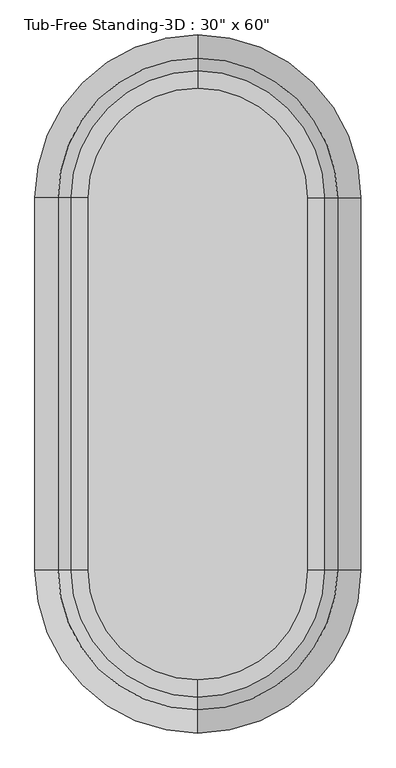
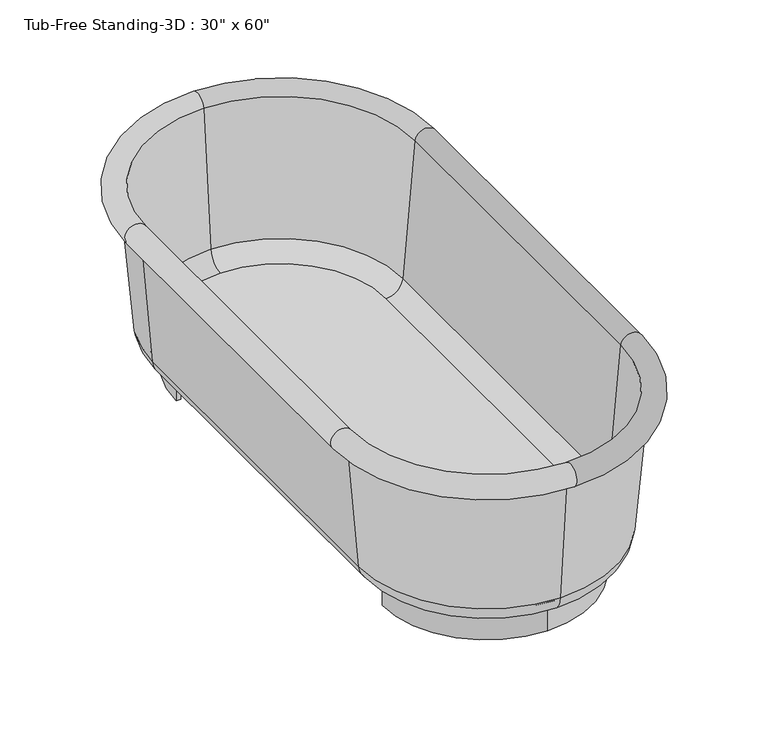
"""IFC4 building model written with IfcOpenShell, lengths in millimetres: flow terminal geometry."""

from ifc_helpers import new_model, si_unit, point, frame, frame_2d, origin, origin_with_axes, place, context, project, spatial, polyline, circle_curve, ellipse_curve, trimmed, segment, composite_curve, outline, extrude, source, transform, mapped, element, save
from ifc_brep_helpers import plane_surface, cylinder_surface, revolved_surface, advanced_brep


def flow_terminal_9fc66f1c(model_context):
    return source(origin(), model_context, "Body", "SolidModel", [
        extrude(outline(composite_curve([segment(trimmed(circle_curve(frame_2d((0.0, 406.4)), 228.6), [point((0.0, 635.0))], [point((-228.6, 406.4))], True, "CARTESIAN"), True, "CONTINUOUS"), segment(polyline([(-228.6, 406.4), (-238.8824236, 406.4)]), True, "CONTINUOUS"), segment(trimmed(circle_curve(frame_2d((0.0, 406.4)), 238.8824236), [point((-238.8824236, 406.4))], [point((0.0, 645.2824236))], False, "CARTESIAN"), True, "CONTINUOUS"), segment(trimmed(circle_curve(frame_2d((0.0, 406.4)), 238.8824236), [point((0.0, 645.2824236))], [point((238.8824236, 406.4))], False, "CARTESIAN"), True, "CONTINUOUS"), segment(polyline([(238.8824236, 406.4), (228.6, 406.4)]), True, "CONTINUOUS"), segment(trimmed(circle_curve(frame_2d((0.0, 406.4)), 228.6), [point((228.6, 406.4))], [point((0.0, 635.0))], True, "CARTESIAN"), True, "CONTINUOUS")], self_intersect=False)), origin_with_axes(), (0.0, 0.0, 1.0), 63.5),
        extrude(outline(composite_curve([segment(trimmed(circle_curve(frame_2d((0.0, -406.4)), 238.8824236), [point((0.0, -645.2824236))], [point((-238.8824236, -406.4))], False, "CARTESIAN"), True, "CONTINUOUS"), segment(polyline([(-238.8824236, -406.4), (-228.6, -406.4)]), True, "CONTINUOUS"), segment(trimmed(circle_curve(frame_2d((0.0, -406.4)), 228.6), [point((-228.6, -406.4))], [point((0.0, -635.0))], True, "CARTESIAN"), True, "CONTINUOUS"), segment(trimmed(circle_curve(frame_2d((0.0, -406.4)), 228.6), [point((0.0, -635.0))], [point((228.6, -406.4))], True, "CARTESIAN"), True, "CONTINUOUS"), segment(polyline([(228.6, -406.4), (238.8824236, -406.4)]), True, "CONTINUOUS"), segment(trimmed(circle_curve(frame_2d((0.0, -406.4)), 238.8824236), [point((238.8824236, -406.4))], [point((0.0, -645.2824236))], False, "CARTESIAN"), True, "CONTINUOUS")], self_intersect=False)), origin_with_axes(), (0.0, 0.0, 1.0), 63.5),
        extrude(outline(composite_curve([segment(polyline([(-238.8824236, -406.4), (-238.8824236, 406.4)]), True, "CONTINUOUS"), segment(trimmed(circle_curve(frame_2d((0.0, 406.4)), 238.8824236), [point((-238.8824236, 406.4))], [point((0.0, 645.2824236))], False, "CARTESIAN"), True, "CONTINUOUS"), segment(trimmed(circle_curve(frame_2d((0.0, 406.4)), 238.8824236), [point((0.0, 645.2824236))], [point((238.8824236, 406.4))], False, "CARTESIAN"), True, "CONTINUOUS"), segment(polyline([(238.8824236, 406.4), (238.8824236, -406.4)]), True, "CONTINUOUS"), segment(trimmed(circle_curve(frame_2d((0.0, -406.4)), 238.8824236), [point((238.8824236, -406.4))], [point((0.0, -645.2824236))], False, "CARTESIAN"), True, "CONTINUOUS"), segment(trimmed(circle_curve(frame_2d((0.0, -406.4)), 238.8824236), [point((0.0, -645.2824236))], [point((-238.8824236, -406.4))], False, "CARTESIAN"), True, "CONTINUOUS")], self_intersect=False)), frame((0.0, 0.0, 63.5), z_axis=(0.0, 0.0, 1.0), x_axis=(1.0, 0.0, 0.0)), (0.0, 0.0, 1.0), 15.08125),
        advanced_brep(
        [(0.0, -723.9, 406.4), (317.5, -406.4, 406.4), (330.2, -406.4, 406.4), (0.0, -736.6, 406.4), (0.0, -698.1045038, 111.5561295), (291.7045038, -406.4, 111.5561295), (0.0, -645.2824236, 63.1536107), (238.8824236, -406.4, 63.1536107), (0.0, -645.2824236, 78.0774627), (238.8824236, -406.4, 78.0774627), (0.0, -683.2374416, 112.8568289), (276.8374416, -406.4, 112.8568289), (0.0, -711.4561556, 435.3982063), (305.0561556, -406.4, 435.3982063), (-317.5, -406.4, 406.4), (-330.2, -406.4, 406.4), (-291.7045038, -406.4, 111.5561295), (-238.8824236, -406.4, 63.1536107), (-238.8824236, -406.4, 78.0774627), (-276.8374416, -406.4, 112.8568289), (-305.0561556, -406.4, 435.3982063), (-330.2, 406.4, 406.4), (-317.5, 406.4, 406.4), (-291.7045038, 406.4, 111.5561295), (-238.8824236, 406.4, 63.1536107), (-238.8824236, 406.4, 78.0774627), (-276.8374416, 406.4, 112.8568289), (-305.0561556, 406.4, 435.3982063), (0.0, 723.9, 406.4), (0.0, 736.6, 406.4), (0.0, 698.1045038, 111.5561295), (0.0, 645.2824236, 63.1536107), (0.0, 645.2824236, 78.0774627), (0.0, 683.2374416, 112.8568289), (0.0, 711.4561556, 435.3982063), (317.5, 406.4, 406.4), (330.2, 406.4, 406.4), (291.7045038, 406.4, 111.5561295), (238.8824236, 406.4, 63.1536107), (238.8824236, 406.4, 78.0774627), (276.8374416, 406.4, 112.8568289), (305.0561556, 406.4, 435.3982063)],
        [
            (0, 1, circle_curve(frame((0.0, -406.4, 406.4), z_axis=(0.0, 0.0, 1.0), x_axis=(1.0, 0.0, 0.0)), 317.5)),
            (1, 2),
            (2, 3, circle_curve(frame((0.0, -406.4, 406.4), z_axis=(0.0, 0.0, -1.0), x_axis=(1.0, 0.0, 0.0)), 330.2)),
            (3, 0),
            (4, 5, circle_curve(frame((0.0, -406.4, 111.5561295), z_axis=(0.0, 0.0, 1.0), x_axis=(1.0, 0.0, 0.0)), 291.7045038)),
            (5, 1),
            (0, 4),
            (6, 7, circle_curve(frame((0.0, -406.4, 63.1536107), z_axis=(0.0, 0.0, 1.0), x_axis=(1.0, 0.0, 0.0)), 238.8824236)),
            (7, 5, circle_curve(frame((238.8824236, -406.4, 116.1774627), z_axis=(0.0, -1.0, 0.0), x_axis=(1.0, 0.0, 0.0)), 53.023852)),
            (4, 6, circle_curve(frame((0.0, -645.2824236, 116.1774627), z_axis=(1.0, 0.0, 0.0), x_axis=(0.0, -1.0, 0.0)), 53.023852)),
            (8, 9, circle_curve(frame((0.0, -406.4, 78.0774627), z_axis=(0.0, 0.0, 1.0), x_axis=(1.0, 0.0, 0.0)), 238.8824236)),
            (9, 7),
            (6, 8),
            (10, 11, circle_curve(frame((0.0, -406.4, 112.8568289), z_axis=(0.0, 0.0, 1.0), x_axis=(1.0, 0.0, 0.0)), 276.8374416)),
            (11, 9, circle_curve(frame((238.8824236, -406.4, 116.1774627), z_axis=(0.0, 1.0, 0.0), x_axis=(1.0, 0.0, 0.0)), 38.1)),
            (8, 10, circle_curve(frame((0.0, -645.2824236, 116.1774627), z_axis=(-1.0, 0.0, 0.0), x_axis=(0.0, -1.0, 0.0)), 38.1)),
            (12, 13, circle_curve(frame((0.0, -406.4, 435.3982063), z_axis=(0.0, 0.0, 1.0), x_axis=(1.0, 0.0, 0.0)), 305.0561556)),
            (13, 11),
            (10, 12),
            (2, 13, circle_curve(frame((330.2, -406.4, 431.8), z_axis=(0.0, -1.0, 0.0), x_axis=(1.0, 0.0, 0.0)), 25.4)),
            (12, 3, circle_curve(frame((0.0, -736.6, 431.8), z_axis=(1.0, 0.0, 0.0), x_axis=(0.0, -1.0, 0.0)), 25.4)),
            (14, 0, circle_curve(frame((0.0, -406.4, 406.4), z_axis=(0.0, 0.0, 1.0), x_axis=(0.0, -1.0, 0.0)), 317.5)),
            (3, 15, circle_curve(frame((0.0, -406.4, 406.4), z_axis=(0.0, 0.0, -1.0), x_axis=(0.0, -1.0, 0.0)), 330.2)),
            (15, 14),
            (16, 4, circle_curve(frame((0.0, -406.4, 111.5561295), z_axis=(0.0, 0.0, 1.0), x_axis=(0.0, -1.0, 0.0)), 291.7045038)),
            (14, 16),
            (17, 6, circle_curve(frame((0.0, -406.4, 63.1536107), z_axis=(0.0, 0.0, 1.0), x_axis=(0.0, -1.0, 0.0)), 238.8824236)),
            (16, 17, circle_curve(frame((-238.8824236, -406.4, 116.1774627), z_axis=(0.0, -1.0, 0.0), x_axis=(-1.0, 0.0, 0.0)), 53.023852)),
            (18, 8, circle_curve(frame((0.0, -406.4, 78.0774627), z_axis=(0.0, 0.0, 1.0), x_axis=(0.0, -1.0, 0.0)), 238.8824236)),
            (17, 18),
            (19, 10, circle_curve(frame((0.0, -406.4, 112.8568289), z_axis=(0.0, 0.0, 1.0), x_axis=(0.0, -1.0, 0.0)), 276.8374416)),
            (18, 19, circle_curve(frame((-238.8824236, -406.4, 116.1774627), z_axis=(0.0, 1.0, 0.0), x_axis=(-1.0, 0.0, 0.0)), 38.1)),
            (20, 12, circle_curve(frame((0.0, -406.4, 435.3982063), z_axis=(0.0, 0.0, 1.0), x_axis=(0.0, -1.0, 0.0)), 305.0561556)),
            (19, 20),
            (20, 15, circle_curve(frame((-330.2, -406.4, 431.8), z_axis=(0.0, -1.0, 0.0), x_axis=(-1.0, 0.0, 0.0)), 25.4)),
            (15, 21),
            (21, 22),
            (22, 14),
            (22, 23),
            (23, 16),
            (23, 24, circle_curve(frame((-238.8824236, 406.4, 116.1774627), z_axis=(0.0, -1.0, 0.0), x_axis=(-1.0, 0.0, 0.0)), 53.023852)),
            (24, 17),
            (24, 25),
            (25, 18),
            (25, 26, circle_curve(frame((-238.8824236, 406.4, 116.1774627), z_axis=(0.0, 1.0, 0.0), x_axis=(-1.0, 0.0, 0.0)), 38.1)),
            (26, 19),
            (26, 27),
            (27, 20),
            (27, 21, circle_curve(frame((-330.2, 406.4, 431.8), z_axis=(0.0, -1.0, 0.0), x_axis=(-1.0, 0.0, 0.0)), 25.4)),
            (28, 22, circle_curve(frame((0.0, 406.4, 406.4), z_axis=(0.0, 0.0, 1.0), x_axis=(-1.0, 0.0, 0.0)), 317.5)),
            (21, 29, circle_curve(frame((0.0, 406.4, 406.4), z_axis=(0.0, 0.0, -1.0), x_axis=(-1.0, 0.0, 0.0)), 330.2)),
            (29, 28),
            (30, 23, circle_curve(frame((0.0, 406.4, 111.5561295), z_axis=(0.0, 0.0, 1.0), x_axis=(-1.0, 0.0, 0.0)), 291.7045038)),
            (28, 30),
            (31, 24, circle_curve(frame((0.0, 406.4, 63.1536107), z_axis=(0.0, 0.0, 1.0), x_axis=(-1.0, 0.0, 0.0)), 238.8824236)),
            (30, 31, circle_curve(frame((0.0, 645.2824236, 116.1774627), z_axis=(-1.0, 0.0, 0.0), x_axis=(0.0, 1.0, 0.0)), 53.023852)),
            (32, 25, circle_curve(frame((0.0, 406.4, 78.0774627), z_axis=(0.0, 0.0, 1.0), x_axis=(-1.0, 0.0, 0.0)), 238.8824236)),
            (31, 32),
            (33, 26, circle_curve(frame((0.0, 406.4, 112.8568289), z_axis=(0.0, 0.0, 1.0), x_axis=(-1.0, 0.0, 0.0)), 276.8374416)),
            (32, 33, circle_curve(frame((0.0, 645.2824236, 116.1774627), z_axis=(1.0, 0.0, 0.0), x_axis=(0.0, 1.0, 0.0)), 38.1)),
            (34, 27, circle_curve(frame((0.0, 406.4, 435.3982063), z_axis=(0.0, 0.0, 1.0), x_axis=(-1.0, 0.0, 0.0)), 305.0561556)),
            (33, 34),
            (34, 29, circle_curve(frame((0.0, 736.6, 431.8), z_axis=(-1.0, 0.0, 0.0), x_axis=(0.0, 1.0, 0.0)), 25.4)),
            (35, 28, circle_curve(frame((0.0, 406.4, 406.4), z_axis=(0.0, 0.0, 1.0), x_axis=(0.0, 1.0, 0.0)), 317.5)),
            (29, 36, circle_curve(frame((0.0, 406.4, 406.4), z_axis=(0.0, 0.0, -1.0), x_axis=(0.0, 1.0, 0.0)), 330.2)),
            (36, 35),
            (37, 30, circle_curve(frame((0.0, 406.4, 111.5561295), z_axis=(0.0, 0.0, 1.0), x_axis=(0.0, 1.0, 0.0)), 291.7045038)),
            (35, 37),
            (38, 31, circle_curve(frame((0.0, 406.4, 63.1536107), z_axis=(0.0, 0.0, 1.0), x_axis=(0.0, 1.0, 0.0)), 238.8824236)),
            (37, 38, circle_curve(frame((238.8824236, 406.4, 116.1774627), z_axis=(0.0, 1.0, 0.0), x_axis=(1.0, 0.0, 0.0)), 53.023852)),
            (39, 32, circle_curve(frame((0.0, 406.4, 78.0774627), z_axis=(0.0, 0.0, 1.0), x_axis=(0.0, 1.0, 0.0)), 238.8824236)),
            (38, 39),
            (40, 33, circle_curve(frame((0.0, 406.4, 112.8568289), z_axis=(0.0, 0.0, 1.0), x_axis=(0.0, 1.0, 0.0)), 276.8374416)),
            (39, 40, circle_curve(frame((238.8824236, 406.4, 116.1774627), z_axis=(0.0, -1.0, 0.0), x_axis=(1.0, 0.0, 0.0)), 38.1)),
            (41, 34, circle_curve(frame((0.0, 406.4, 435.3982063), z_axis=(0.0, 0.0, 1.0), x_axis=(0.0, 1.0, 0.0)), 305.0561556)),
            (40, 41),
            (41, 36, circle_curve(frame((330.2, 406.4, 431.8), z_axis=(0.0, 1.0, 0.0), x_axis=(1.0, 0.0, 0.0)), 25.4)),
            (36, 2),
            (1, 35),
            (5, 37),
            (7, 38),
            (9, 39),
            (11, 40),
            (13, 41),
        ],
        [
            plane_surface(frame((0.0, -406.4, 406.4), z_axis=(0.0, 0.0, -1.0), x_axis=(1.0, 0.0, 0.0))),
            revolved_surface(polyline([(317.5, -406.4, 406.4), (291.7045038, -406.4, 111.5561295)]), (0.0, -406.4, 431.8), (0.0, 0.0, -1.0)),
            revolved_surface(trimmed(ellipse_curve(frame((238.8824236, -406.4, 116.1774627), z_axis=(0.0, 1.0, 0.0), x_axis=(1.0, 0.0, 0.0)), 53.023852, 53.023852), [point((291.7045038, -406.4, 111.5561295))], [point((238.8824236, -406.4, 63.1536107))], True, "CARTESIAN"), (0.0, -406.4, 431.8), (0.0, 0.0, -1.0)),
            revolved_surface(polyline([(238.8824236, -406.4, 63.1536107), (238.8824236, -406.4, 78.07746270000001)]), (0.0, -406.4, 431.8), (0.0, 0.0, -1.0)),
            revolved_surface(trimmed(ellipse_curve(frame((238.8824236, -406.4, 116.1774627), z_axis=(0.0, -1.0, 0.0), x_axis=(1.0, 0.0, 0.0)), 38.1, 38.1), [point((238.8824236, -406.4, 78.0774627))], [point((276.8374416, -406.4, 112.8568289))], True, "CARTESIAN"), (0.0, -406.4, 431.8), (0.0, 0.0, -1.0)),
            revolved_surface(polyline([(276.8374416, -406.4, 112.8568289), (305.0561556, -406.4, 435.3982063)]), (0.0, -406.4, 431.8), (0.0, 0.0, -1.0)),
            revolved_surface(trimmed(ellipse_curve(frame((330.2, -406.4, 431.8), z_axis=(0.0, 1.0, 0.0), x_axis=(1.0, 0.0, 0.0)), 25.4, 25.4), [point((305.0561556, -406.4, 435.3982063))], [point((330.2, -406.4, 406.4))], True, "CARTESIAN"), (0.0, -406.4, 431.8), (0.0, 0.0, -1.0)),
            plane_surface(frame((0.0, -406.4, 406.4), z_axis=(0.0, 0.0, -1.0), x_axis=(0.0, -1.0, 0.0))),
            revolved_surface(polyline([(0.0, -723.9, 406.4), (0.0, -698.1045038, 111.5561295)]), (0.0, -406.4, 431.8), (0.0, 0.0, -1.0)),
            revolved_surface(trimmed(ellipse_curve(frame((0.0, -645.2824236, 116.1774627), z_axis=(1.0, 0.0, 0.0), x_axis=(0.0, -1.0, 0.0)), 53.023852, 53.023852), [point((0.0, -698.1045038, 111.5561295))], [point((0.0, -645.2824236, 63.1536107))], True, "CARTESIAN"), (0.0, -406.4, 431.8), (0.0, 0.0, -1.0)),
            revolved_surface(polyline([(0.0, -645.2824236, 63.1536107), (0.0, -645.2824236, 78.07746270000001)]), (0.0, -406.4, 431.8), (0.0, 0.0, -1.0)),
            revolved_surface(trimmed(ellipse_curve(frame((0.0, -645.2824236, 116.1774627), z_axis=(-1.0, 0.0, 0.0), x_axis=(0.0, -1.0, 0.0)), 38.1, 38.1), [point((0.0, -645.2824236, 78.0774627))], [point((0.0, -683.2374416, 112.8568289))], True, "CARTESIAN"), (0.0, -406.4, 431.8), (0.0, 0.0, -1.0)),
            revolved_surface(polyline([(0.0, -683.2374416, 112.8568289), (0.0, -711.4561556, 435.3982063)]), (0.0, -406.4, 431.8), (0.0, 0.0, -1.0)),
            revolved_surface(trimmed(ellipse_curve(frame((0.0, -736.6, 431.8), z_axis=(1.0, 0.0, 0.0), x_axis=(0.0, -1.0, 0.0)), 25.4, 25.4), [point((0.0, -711.4561556, 435.3982063))], [point((0.0, -736.6, 406.4))], True, "CARTESIAN"), (0.0, -406.4, 431.8), (0.0, 0.0, -1.0)),
            plane_surface(frame((-330.2, -406.4, 406.4), z_axis=(0.0, 0.0, -1.0), x_axis=(0.0, 1.0, 0.0))),
            plane_surface(frame((-317.5, -406.4, 406.4), z_axis=(-0.9961946980917455, 0.0, -0.08715574274765882), x_axis=(0.0, 1.0, 0.0))),
            cylinder_surface(frame((-238.8824236, -406.4, 116.1774627), z_axis=(0.0, -1.0, 0.0), x_axis=(-1.0, 0.0, 0.0)), 53.023852),
            plane_surface(frame((-238.8824236, -406.4, 63.1536107), z_axis=(1.0, 0.0, 0.0), x_axis=(0.0, 1.0, 0.0))),
            revolved_surface(polyline([(-276.9824236, 406.4, 116.1774627), (-276.9824236, -406.4, 116.1774627)]), (-238.8824236, -406.4, 116.1774627), (0.0, 1.0, 0.0)),
            plane_surface(frame((-276.8374416, -406.4, 112.8568289), z_axis=(0.9961946980917457, 0.0, 0.08715574274765688), x_axis=(0.0, 1.0, 0.0))),
            cylinder_surface(frame((-330.2, -406.4, 431.8), z_axis=(0.0, -1.0, 0.0), x_axis=(-1.0, 0.0, 0.0)), 25.4),
            plane_surface(frame((0.0, 406.4, 406.4), z_axis=(0.0, 0.0, -1.0), x_axis=(-1.0, 0.0, 0.0))),
            revolved_surface(polyline([(-317.5, 406.4, 406.4), (-291.7045038, 406.4, 111.5561295)]), (0.0, 406.4, 431.8), (0.0, 0.0, -1.0)),
            revolved_surface(trimmed(ellipse_curve(frame((-238.8824236, 406.4, 116.1774627), z_axis=(0.0, -1.0, 0.0), x_axis=(-1.0, 0.0, 0.0)), 53.023852, 53.023852), [point((-291.7045038, 406.4, 111.5561295))], [point((-238.8824236, 406.4, 63.1536107))], True, "CARTESIAN"), (0.0, 406.4, 431.8), (0.0, 0.0, -1.0)),
            revolved_surface(polyline([(-238.8824236, 406.4, 63.1536107), (-238.8824236, 406.4, 78.07746270000001)]), (0.0, 406.4, 431.8), (0.0, 0.0, -1.0)),
            revolved_surface(trimmed(ellipse_curve(frame((-238.8824236, 406.4, 116.1774627), z_axis=(0.0, 1.0, 0.0), x_axis=(-1.0, 0.0, 0.0)), 38.1, 38.1), [point((-238.8824236, 406.4, 78.0774627))], [point((-276.8374416, 406.4, 112.8568289))], True, "CARTESIAN"), (0.0, 406.4, 431.8), (0.0, 0.0, -1.0)),
            revolved_surface(polyline([(-276.8374416, 406.4, 112.8568289), (-305.0561556, 406.4, 435.3982063)]), (0.0, 406.4, 431.8), (0.0, 0.0, -1.0)),
            revolved_surface(trimmed(ellipse_curve(frame((-330.2, 406.4, 431.8), z_axis=(0.0, -1.0, 0.0), x_axis=(-1.0, 0.0, 0.0)), 25.4, 25.4), [point((-305.0561556, 406.4, 435.3982063))], [point((-330.2, 406.4, 406.4))], True, "CARTESIAN"), (0.0, 406.4, 431.8), (0.0, 0.0, -1.0)),
            plane_surface(frame((0.0, 406.4, 406.4), z_axis=(0.0, 0.0, -1.0), x_axis=(0.0, 1.0, 0.0))),
            revolved_surface(polyline([(0.0, 723.9, 406.4), (0.0, 698.1045038, 111.5561295)]), (0.0, 406.4, 431.8), (0.0, 0.0, -1.0)),
            revolved_surface(trimmed(ellipse_curve(frame((0.0, 645.2824236, 116.1774627), z_axis=(-1.0, 0.0, 0.0), x_axis=(0.0, 1.0, 0.0)), 53.023852, 53.023852), [point((0.0, 698.1045038, 111.5561295))], [point((0.0, 645.2824236, 63.1536107))], True, "CARTESIAN"), (0.0, 406.4, 431.8), (0.0, 0.0, -1.0)),
            revolved_surface(polyline([(0.0, 645.2824236, 63.1536107), (0.0, 645.2824236, 78.07746270000001)]), (0.0, 406.4, 431.8), (0.0, 0.0, -1.0)),
            revolved_surface(trimmed(ellipse_curve(frame((0.0, 645.2824236, 116.1774627), z_axis=(1.0, 0.0, 0.0), x_axis=(0.0, 1.0, 0.0)), 38.1, 38.1), [point((0.0, 645.2824236, 78.0774627))], [point((0.0, 683.2374416, 112.8568289))], True, "CARTESIAN"), (0.0, 406.4, 431.8), (0.0, 0.0, -1.0)),
            revolved_surface(polyline([(0.0, 683.2374416, 112.8568289), (0.0, 711.4561556, 435.3982063)]), (0.0, 406.4, 431.8), (0.0, 0.0, -1.0)),
            revolved_surface(trimmed(ellipse_curve(frame((0.0, 736.6, 431.8), z_axis=(-1.0, 0.0, 0.0), x_axis=(0.0, 1.0, 0.0)), 25.4, 25.4), [point((0.0, 711.4561556, 435.3982063))], [point((0.0, 736.6, 406.4))], True, "CARTESIAN"), (0.0, 406.4, 431.8), (0.0, 0.0, -1.0)),
            plane_surface(frame((330.2, 406.4, 406.4), z_axis=(0.0, 0.0, -1.0), x_axis=(0.0, -1.0, 0.0))),
            plane_surface(frame((317.5, 406.4, 406.4), z_axis=(0.9961946980917455, 0.0, -0.08715574274765882), x_axis=(0.0, -1.0, 0.0))),
            cylinder_surface(frame((238.8824236, 406.4, 116.1774627), z_axis=(0.0, 1.0, 0.0), x_axis=(1.0, 0.0, 0.0)), 53.023852),
            plane_surface(frame((238.8824236, 406.4, 63.1536107), z_axis=(-1.0, 0.0, 0.0), x_axis=(0.0, -1.0, 0.0))),
            revolved_surface(polyline([(276.9824236, -406.4, 116.1774627), (276.9824236, 406.4, 116.1774627)]), (238.8824236, 406.4, 116.1774627), (0.0, -1.0, 0.0)),
            plane_surface(frame((276.8374416, 406.4, 112.8568289), z_axis=(-0.9961946980917458, 0.0, 0.08715574274765689), x_axis=(0.0, -1.0, 0.0))),
            cylinder_surface(frame((330.2, 406.4, 431.8), z_axis=(0.0, 1.0, 0.0), x_axis=(1.0, 0.0, 0.0)), 25.4),
        ],
        [
            (0, [[1, 2, 3, 4]]),
            (1, [[5, 6, -1, 7]]),
            (2, [[8, 9, -5, 10]]),
            (3, [[11, 12, -8, 13]]),
            (4, [[14, 15, -11, 16]]),
            (5, [[17, 18, -14, 19]]),
            (6, [[-3, 20, -17, 21]]),
            (7, [[22, -4, 23, 24]]),
            (8, [[25, -7, -22, 26]]),
            (9, [[27, -10, -25, 28]]),
            (10, [[29, -13, -27, 30]]),
            (11, [[31, -16, -29, 32]]),
            (12, [[33, -19, -31, 34]]),
            (13, [[-23, -21, -33, 35]]),
            (14, [[-24, 36, 37, 38]]),
            (15, [[-26, -38, 39, 40]]),
            (16, [[-28, -40, 41, 42]]),
            (17, [[-30, -42, 43, 44]]),
            (18, [[-32, -44, 45, 46]]),
            (19, [[-34, -46, 47, 48]]),
            (20, [[-35, -48, 49, -36]]),
            (21, [[50, -37, 51, 52]]),
            (22, [[53, -39, -50, 54]]),
            (23, [[55, -41, -53, 56]]),
            (24, [[57, -43, -55, 58]]),
            (25, [[59, -45, -57, 60]]),
            (26, [[61, -47, -59, 62]]),
            (27, [[-51, -49, -61, 63]]),
            (28, [[64, -52, 65, 66]]),
            (29, [[67, -54, -64, 68]]),
            (30, [[69, -56, -67, 70]]),
            (31, [[71, -58, -69, 72]]),
            (32, [[73, -60, -71, 74]]),
            (33, [[75, -62, -73, 76]]),
            (34, [[-65, -63, -75, 77]]),
            (35, [[-66, 78, -2, 79]]),
            (36, [[-68, -79, -6, 80]]),
            (37, [[-70, -80, -9, 81]]),
            (38, [[-72, -81, -12, 82]]),
            (39, [[-74, -82, -15, 83]]),
            (40, [[-76, -83, -18, 84]]),
            (41, [[-77, -84, -20, -78]]),
        ],
    ),
    ])


if __name__ == "__main__":
    model = new_model("IFC4")
    model_context = context("Model", 3, world=origin())
    ifc_project = project(units=[si_unit("LENGTHUNIT", "METRE", prefix="MILLI")], contexts=[model_context])
    site = spatial("IfcSite", under=ifc_project)
    building = spatial("IfcBuilding", under=site)
    placement = place(None, origin())
    flow_terminal_shape = flow_terminal_9fc66f1c(model_context)
    element("IfcFlowTerminal", 1, ObjectType="Tub-Free Standing-3D : 30\" x 60\"", at=placement, inside=building, context=model_context, shape_type="MappedRepresentation", body=[
        mapped(flow_terminal_shape, transform((0.0, 0.0, 0.0), x_axis=(1.0, 0.0, 0.0), y_axis=(0.0, 1.0, 0.0), z_axis=(0.0, 0.0, 1.0))),
    ])
    save(model, "model.ifc")

# Revit data of these elements
# Type "Tub-Free Standing-3D : 30\" x 60\""
#   Assembly Code = "D2010110"
#   Height = 1' - 6"
#   Length = 5' - 0"
#   Width = 2' - 4"
#   Tub Material = Porcelain, Ivory
#   Default Elevation = 0
# Element 1 (IfcFlowTerminal, "Tub-Free Standing-3D : 30\" x 60\"")
#   Materials on its faces: "Porcelain, Ivory"
# Materials
#   "Porcelain, Ivory": class "Ceramic", colour RGB 247 247 239, transparency 0, Description = "Porcelain, ivory", Cost = 0
